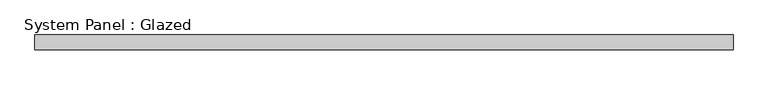
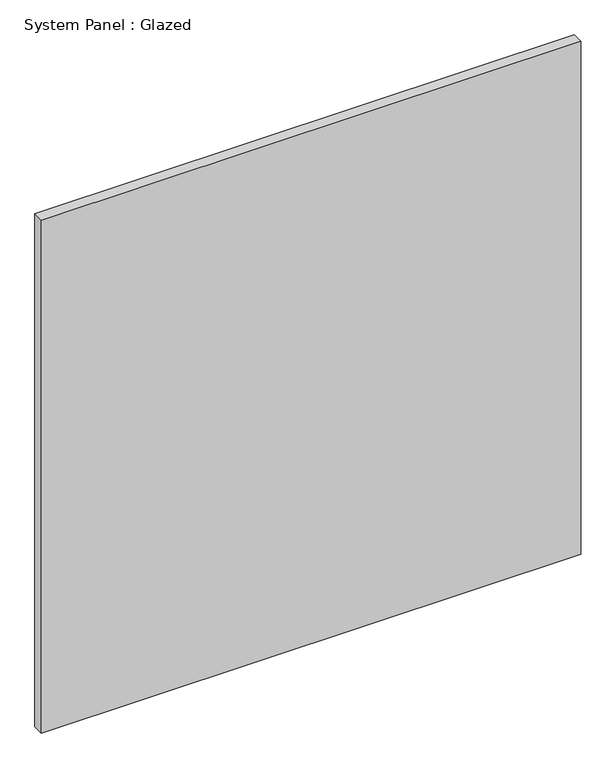
"""IFC4 building model written with IfcOpenShell, lengths in millimetres: plate geometry, System Panel : Glazed."""

from ifc_helpers import new_model, si_unit, origin, origin_with_axes, place, context, project, spatial, polyline, outline, extrude, source, transform, mapped, element, save


def system_panel_glazed_dd75d2a7(model_context):
    return source(origin(), model_context, "Body", "SweptSolid", [
        extrude(outline(polyline([(596.6666667, 24.5), (-596.6666667, 24.5), (-596.6666667, 49.5), (596.6666667, 49.5), (596.6666667, 24.5)])), origin_with_axes(), (0.0, 0.0, 1.0), 1200.0),
    ])


if __name__ == "__main__":
    model = new_model("IFC4")
    model_context = context("Model", 3, world=origin())
    ifc_project = project(units=[si_unit("LENGTHUNIT", "METRE", prefix="MILLI")], contexts=[model_context])
    site = spatial("IfcSite", under=ifc_project)
    building = spatial("IfcBuilding", under=site)
    placement = place(None, origin())
    system_panel_glazed_shape = system_panel_glazed_dd75d2a7(model_context)
    element("IfcPlate", 1, ObjectType="System Panel : Glazed", at=placement, inside=building, context=model_context, shape_type="MappedRepresentation", body=[
        mapped(system_panel_glazed_shape, transform((0.0, 0.0, 0.0), x_axis=(1.0, 0.0, 0.0), y_axis=(0.0, 1.0, 0.0), z_axis=(0.0, 0.0, 1.0))),
    ])
    save(model, "model.ifc")

# Revit data of these elements
# Type "System Panel : Glazed"
#   Keynote = "H11"
#   Construction Type Id = "GSP4R"
#   Analytic Construction = "1/8 in Pilkington single glazing"
#   Visual Light Transmittance = 0.9
#   Solar Heat Gain Coefficient = 0.86
#   Heat Transfer Coefficient (U) = 6.7069 W/(m²·K)
#   Define Thermal Properties by = 1
# Element 1 (IfcPlate, "System Panel : Glazed")
#   Materials on its faces: "Glass"
# Materials
#   "Glass": class "Glass", colour RGB 0 128 192, transparency 0.9, Description = "Soda Lime Glass", Cost = 0
